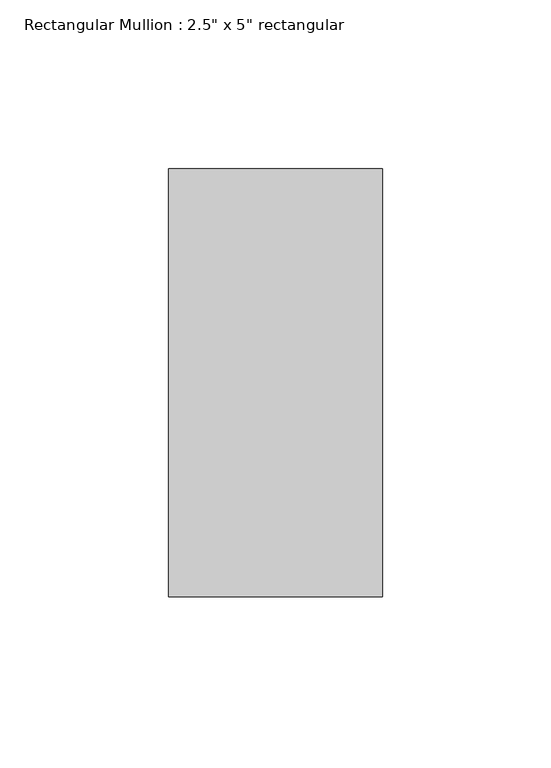
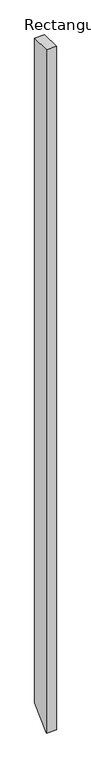
"""IFC4 building model written with IfcOpenShell, lengths in millimetres: member geometry."""

from ifc_helpers import new_model, si_unit, frame, origin, place, context, project, spatial, polyline, outline, extrude, source, transform, mapped, element, save


def member_bee66a91(model_context):
    return source(origin(), model_context, "Body", "SweptSolid", [
        extrude(outline(polyline([(-63.5, 0.0), (63.5, 0.0), (63.5, -4439.2138225), (-63.5, -4566.2138225), (-63.5, 0.0)])), frame((-63.5, 0.0, 0.0), z_axis=(1.0, 0.0, 0.0), x_axis=(0.0, 1.0, 0.0)), (0.0, 0.0, 1.0), 63.5),
    ])


if __name__ == "__main__":
    model = new_model("IFC4")
    model_context = context("Model", 3, world=origin())
    ifc_project = project(units=[si_unit("LENGTHUNIT", "METRE", prefix="MILLI")], contexts=[model_context])
    site = spatial("IfcSite", under=ifc_project)
    building = spatial("IfcBuilding", under=site)
    placement = place(None, origin())
    member_shape = member_bee66a91(model_context)
    element("IfcMember", 1, ObjectType="Rectangular Mullion : 2.5\" x 5\" rectangular", at=placement, inside=building, context=model_context, shape_type="MappedRepresentation", body=[
        mapped(member_shape, transform((0.0, 0.0, 0.0), x_axis=(1.0, 0.0, 0.0), y_axis=(0.0, 1.0, 0.0), z_axis=(0.0, 0.0, 1.0))),
    ])
    save(model, "model.ifc")

# Revit data of these elements
# Type "Rectangular Mullion : 2.5\" x 5\" rectangular"
#   built-in parameter 1007304 = 0.416667 (stored number, unit not read)
#   built-in parameter 1007301 = 0.104167 (stored number, unit not read)
#   built-in parameter 1007300 = 0.104167 (stored number, unit not read)
# Element 1 (IfcMember, "Rectangular Mullion : 2.5\" x 5\" rectangular")
#   Materials on its faces: "Aluminum"
# Materials
#   "Aluminum": class "Metal", colour RGB 247 247 247, transparency 0, Description = "Aluminum 6061", Cost = 0
